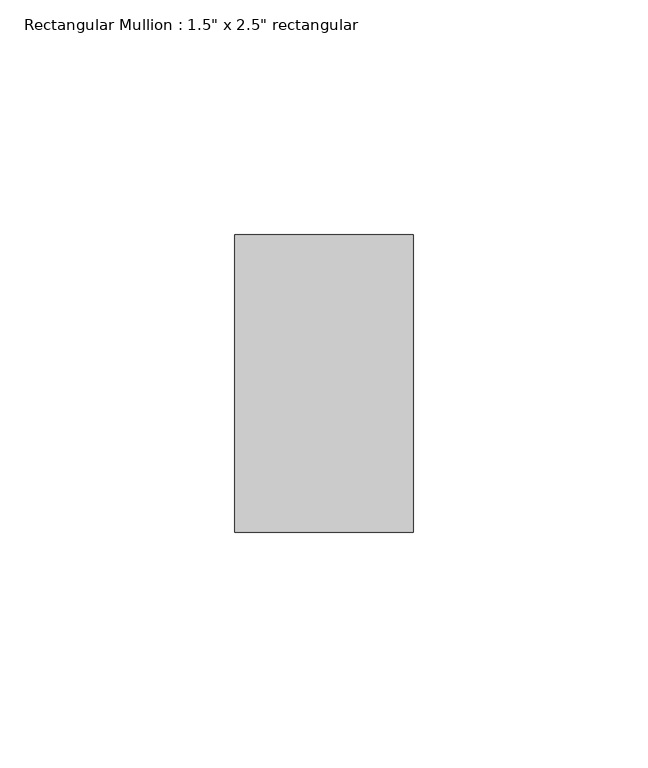
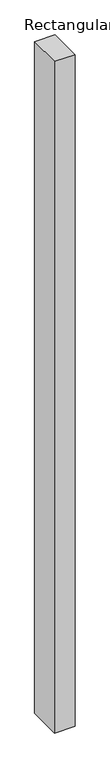
"""IFC4 building model written with IfcOpenShell, lengths in millimetres: member geometry."""

from ifc_helpers import new_model, si_unit, frame, origin, place, context, project, spatial, polyline, outline, extrude, source, transform, mapped, element, save


def member_f8a7f713(model_context):
    return source(origin(), model_context, "Body", "SweptSolid", [
        extrude(outline(polyline([(19.05, 31.75), (19.05, -31.75), (-19.05, -31.75), (-19.05, 31.75), (19.05, 31.75)])), frame((0.0, 0.0, -1315.2360761), z_axis=(0.0, 0.0, 1.0), x_axis=(1.0, 0.0, 0.0)), (0.0, 0.0, 1.0), 1315.2360761),
    ])


if __name__ == "__main__":
    model = new_model("IFC4")
    model_context = context("Model", 3, world=origin())
    ifc_project = project(units=[si_unit("LENGTHUNIT", "METRE", prefix="MILLI")], contexts=[model_context])
    site = spatial("IfcSite", under=ifc_project)
    building = spatial("IfcBuilding", under=site)
    placement = place(None, origin())
    member_shape = member_f8a7f713(model_context)
    element("IfcMember", 1, ObjectType="Rectangular Mullion : 1.5\" x 2.5\" rectangular", at=placement, inside=building, context=model_context, shape_type="MappedRepresentation", body=[
        mapped(member_shape, transform((0.0, 0.0, 0.0), x_axis=(1.0, 0.0, 0.0), y_axis=(0.0, 1.0, 0.0), z_axis=(0.0, 0.0, 1.0))),
    ])
    save(model, "model.ifc")

# Revit data of these elements
# Type "Rectangular Mullion : 1.5\" x 2.5\" rectangular"
#   built-in parameter 1007304 = 0.208333 (stored number, unit not read)
#   built-in parameter 1007301 = 0.0625 (stored number, unit not read)
#   built-in parameter 1007300 = 0.0625 (stored number, unit not read)
# Element 1 (IfcMember, "Rectangular Mullion : 1.5\" x 2.5\" rectangular")
#   Materials on its faces: "Damp-proofing"
# Materials
#   "Damp-proofing": class "Generic", colour RGB 127 127 127, transparency 0, Description = "Damp-proofing", Cost = 0
